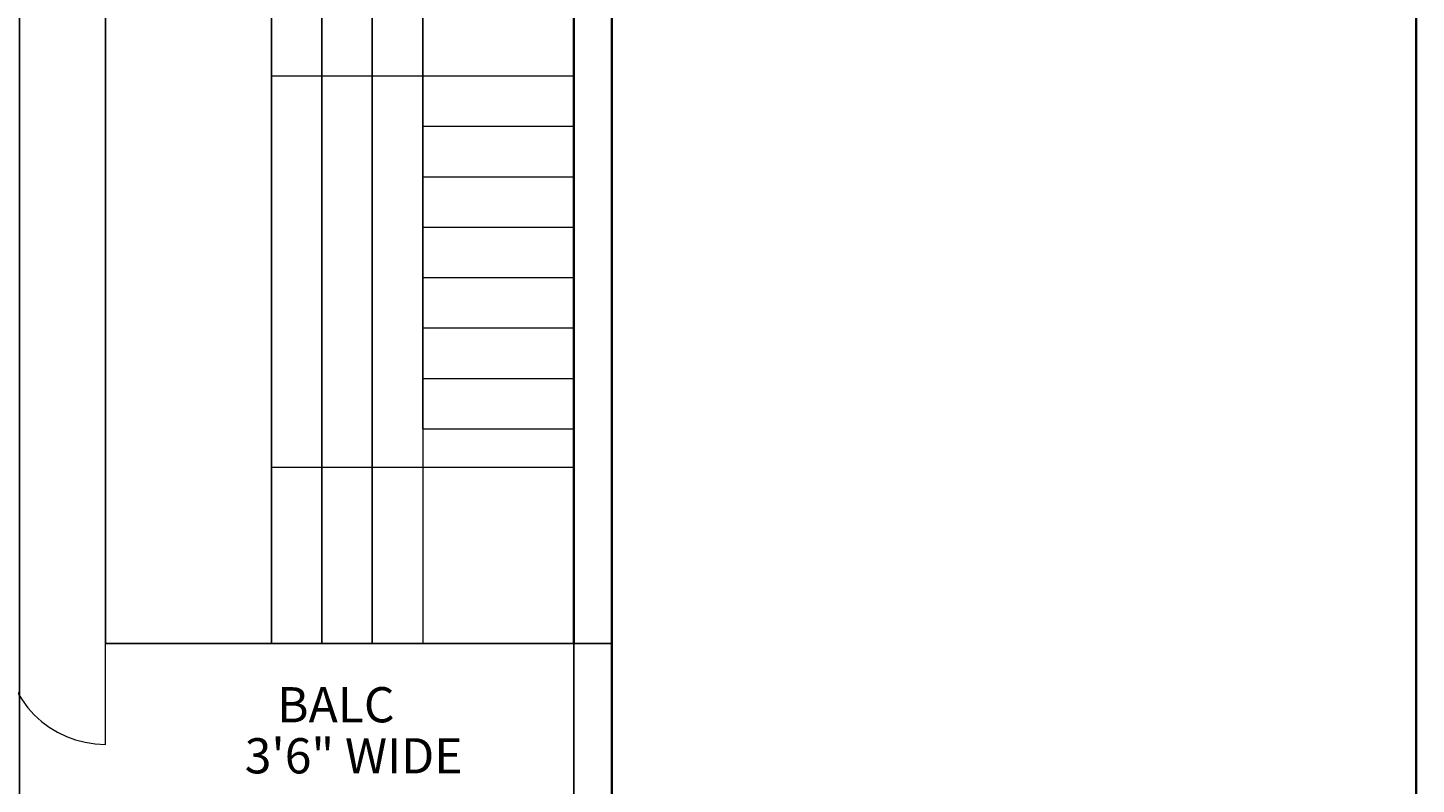
# Model space of a CAD drawing. Units: feet. Extents: x 1654 to 2985, y 1348 to 2230.
# Tile 43 of 53: x 2655 to 2985, y 1532 to 1712. Entities that reach past the tile are written whole.
import ezdxf

# ---------------------------------------------------------------- set-up
doc = ezdxf.new("R2010")
doc.units = ezdxf.units.FT
for name, color, linetype, lineweight in [('A-ANNO-DIMS', 2, 'Continuous', 18), ('A-ANNO-TTLB', 7, 'Continuous', 35), ('A-AREA-IDEN', 7, 'Continuous', 18), ('A-DOOR', 3, 'Continuous', 18), ('A-FLOR', 7, 'Continuous', 25), ('A-FLOR-STRS', 7, 'Continuous', 18), ('A-WALL', 7, 'Continuous', 35)]:
    doc.layers.add(name, color=color, linetype=linetype, lineweight=lineweight)
doc.styles.get("Standard").update_dxf_attribs({"font": 'arial.ttf'})
doc.dimstyles.get("Standard").update_dxf_attribs({"dimtxt": 0.18, "dimasz": 0.18, "dimexe": 0.18, "dimexo": 0.0625, "dimgap": 0.09, "dimtad": 0, "dimtih": 1, "dimtoh": 1, "dimdec": 4, "dimzin": 0, "dimdsep": 46, "dimtxsty": 'Standard', "dimcen": 0.09, "dimadec": 0, "dimazin": 0, "dimtfac": 1, "dimtdec": 4, "dimtofl": 0, "dimtmove": 0, "dimatfit": 3, "dimfxl": 1, "dimtolj": 1, "dimtzin": 0, "dimarcsym": 0})

# ---------------------------------------------------------------- blocks, each defined once
blk = doc.blocks.new('STAIR-RETURN')
for p, q in [((0, 186), (0, 135)), ((36, 186), (36, 0)), ((0, 177), (0, 135)), ((12, 177), (12, 135)), ((12, 177), (12, 135)), ((24, 177), (24, 135)), ((24, 177), (24, 135)), ((72, 135), (0, 135)), ((72, 123), (36, 123)), ((72, 111), (36, 111)), ((72, 99), (36, 99)), ((72, 87), (36, 87)), ((72, 75), (36, 75)), ((72, 63), (36, 63)), ((72, 51), (36, 51)), ((0, 42), (72, 42)), ((0, 42), (0, 0)), ((12, 42), (12, 0)), ((24, 42), (24, 0))]:
    blk.add_line(p, q)
blk = doc.blocks.new('*D82')
at = {"layer": 'A-ANNO-DIMS', "color": 0, "lineweight": -2, "transparency": 16777216}
for p, q in [((2652.71, 2039.19), (2652.71, 1490.62)), ((2784.71, 2039.19), (2784.71, 1490.62)), ((2652.89, 1490.8), (2718.43, 1490.8)), ((2784.53, 1490.8), (2718.99, 1490.8))]:
    blk.add_line(p, q, dxfattribs=at)
at = {"layer": 'A-ANNO-DIMS', "color": 0, "transparency": 16777216}
for points in [[(2652.89, 1490.83), (2652.89, 1490.77), (2652.71, 1490.8)], [(2784.53, 1490.83), (2784.53, 1490.77), (2784.71, 1490.8)]]:
    blk.add_solid(points, dxfattribs=at)
at = {"layer": 'Defpoints', "color": 0, "transparency": 16777216}
for p in [(2652.71, 2039.25), (2784.71, 2039.25), (2784.71, 1490.8)]:
    blk.add_point(p, dxfattribs=at)
at = {"layer": 'A-ANNO-DIMS', "color": 0, "transparency": 16777216, "insert": (2718.71, 1490.8), "char_height": 0.18, "attachment_point": 5}
blk.add_mtext('\\A1;132', dxfattribs=at)
blk = doc.blocks.new('*D84')
at = {"layer": 'A-ANNO-DIMS', "color": 0, "lineweight": -2, "transparency": 16777216}
for p, q in [((2625.24, 1565.32), (2625.24, 2149.88)), ((2625.42, 2149.7), (2649.01, 2149.7)), ((2673.06, 2149.7), (2649.46, 2149.7)), ((2673.24, 1565.32), (2673.24, 2149.88))]:
    blk.add_line(p, q, dxfattribs=at)
at = {"layer": 'A-ANNO-DIMS', "color": 0, "transparency": 16777216}
for points in [[(2625.42, 2149.73), (2625.42, 2149.67), (2625.24, 2149.7)], [(2673.06, 2149.73), (2673.06, 2149.67), (2673.24, 2149.7)]]:
    blk.add_solid(points, dxfattribs=at)
at = {"layer": 'Defpoints', "color": 0, "transparency": 16777216}
for p in [(2673.24, 2149.7), (2625.24, 1565.25), (2673.24, 1565.25)]:
    blk.add_point(p, dxfattribs=at)
at = {"layer": 'A-ANNO-DIMS', "color": 0, "transparency": 16777216, "insert": (2649.24, 2149.7), "char_height": 0.18, "attachment_point": 5}
blk.add_mtext('\\A1;48', dxfattribs=at)
blk = doc.blocks.new('*D85')
at = {"layer": 'A-ANNO-DIMS', "color": 0, "lineweight": -2, "transparency": 16777216}
for p, q in [((2673.24, 1565.32), (2673.24, 2149.88)), ((2673.42, 2149.7), (2692.58, 2149.7)), ((2712.53, 2149.7), (2693.36, 2149.7)), ((2712.71, 1565.32), (2712.71, 2149.88))]:
    blk.add_line(p, q, dxfattribs=at)
at = {"layer": 'A-ANNO-DIMS', "color": 0, "transparency": 16777216}
for points in [[(2673.42, 2149.73), (2673.42, 2149.67), (2673.24, 2149.7)], [(2712.53, 2149.73), (2712.53, 2149.67), (2712.71, 2149.7)]]:
    blk.add_solid(points, dxfattribs=at)
at = {"layer": 'Defpoints', "color": 0, "transparency": 16777216}
for p in [(2712.71, 2149.7), (2673.24, 1565.25), (2712.71, 1565.25)]:
    blk.add_point(p, dxfattribs=at)
at = {"layer": 'A-ANNO-DIMS', "color": 0, "transparency": 16777216, "insert": (2692.97, 2149.7), "char_height": 0.18, "attachment_point": 5}
blk.add_mtext('\\A1;39.47', dxfattribs=at)
blk = doc.blocks.new('*D86')
at = {"layer": 'A-ANNO-DIMS', "color": 0, "lineweight": -2, "transparency": 16777216}
for p, q in [((2748.71, 1616.32), (2748.71, 2149.88)), ((2748.89, 2149.7), (2766.49, 2149.7)), ((2784.53, 2149.7), (2766.92, 2149.7)), ((2784.71, 1607.32), (2784.71, 2149.88))]:
    blk.add_line(p, q, dxfattribs=at)
at = {"layer": 'A-ANNO-DIMS', "color": 0, "transparency": 16777216}
for points in [[(2748.89, 2149.73), (2748.89, 2149.67), (2748.71, 2149.7)], [(2784.53, 2149.73), (2784.53, 2149.67), (2784.71, 2149.7)]]:
    blk.add_solid(points, dxfattribs=at)
at = {"layer": 'Defpoints', "color": 0, "transparency": 16777216}
for p in [(2784.71, 2149.7), (2748.71, 1616.25), (2784.71, 1607.25)]:
    blk.add_point(p, dxfattribs=at)
at = {"layer": 'A-ANNO-DIMS', "color": 0, "transparency": 16777216, "insert": (2766.71, 2149.7), "char_height": 0.18, "attachment_point": 5}
blk.add_mtext('\\A1;36', dxfattribs=at)
blk = doc.blocks.new('*D87')
at = {"layer": 'A-ANNO-DIMS', "color": 0, "lineweight": -2, "transparency": 16777216}
for p, q in [((2724.71, 1565.32), (2724.71, 2149.88)), ((2724.89, 2149.7), (2730.5, 2149.7)), ((2736.53, 2149.7), (2730.92, 2149.7)), ((2736.71, 1565.32), (2736.71, 2149.88))]:
    blk.add_line(p, q, dxfattribs=at)
at = {"layer": 'A-ANNO-DIMS', "color": 0, "transparency": 16777216}
for points in [[(2724.89, 2149.73), (2724.89, 2149.67), (2724.71, 2149.7)], [(2736.53, 2149.73), (2736.53, 2149.67), (2736.71, 2149.7)]]:
    blk.add_solid(points, dxfattribs=at)
at = {"layer": 'Defpoints', "color": 0, "transparency": 16777216}
for p in [(2736.71, 2149.7), (2724.71, 1565.25), (2736.71, 1565.25)]:
    blk.add_point(p, dxfattribs=at)
at = {"layer": 'A-ANNO-DIMS', "color": 0, "transparency": 16777216, "insert": (2730.71, 2149.7), "char_height": 0.18, "attachment_point": 5}
blk.add_mtext('\\A1;12', dxfattribs=at)

msp = doc.modelspace()

# ---------------------------------------------------------------- linework, layer by layer
at = {"layer": 'A-ANNO-TTLB'}
msp.add_lwpolyline([(1654.1997, 2230.0267), (2985.175, 2230.0267), (2985.175, 1348.1324), (1654.1997, 1348.1324)], close=True, dxfattribs=at)
at = {"layer": 'A-DOOR'}
msp.add_line((2673.2353, 1541.2549), (2673.2353, 1565.2549), dxfattribs=at)
msp.add_arc((2673.2353, 1565.2549), 24, 180, 270, dxfattribs=at)
at = {"layer": 'A-FLOR'}
msp.add_line((2673.2353, 1565.2549), (2793.7058, 1565.2549), dxfattribs=at)
at = {"layer": 'A-WALL'}
for p, q in [((2793.7058, 1886.2549), (2793.7058, 1523.2549)), ((2784.7058, 1742.2549), (2784.7058, 1565.2549))]:
    msp.add_line(p, q, dxfattribs=at)

# ---------------------------------------------------------------- block references
at = {"layer": 'A-FLOR-STRS'}
msp.add_blockref('STAIR-RETURN', (2712.7054, 1565.255), dxfattribs=at)

# ---------------------------------------------------------------- texts
at = {"layer": 'A-AREA-IDEN'}
for s, p in [('BALC', (2714.0307, 1546.4962)), ('3\'6" WIDE', (2706.3476, 1534.3486))]:
    msp.add_text(s, height=8.38114, dxfattribs=at).set_placement(p)

# ---------------------------------------------------------------- dimensions: what is measured, and where the dimension line sits
at = {"layer": 'A-ANNO-DIMS'}
for base, p1, p2, override, picture, middle in [((2673.2353, 2149.7049), (2625.2353, 1565.2549), (2673.2353, 1565.2549), {"dimdec": 0, "dimlfac": 1, "dimrnd": 0, "dimzin": 0, "dimdsep": 46, "dimlunit": 2}, '*D84', (2649.2353, 2149.7049)), ((2712.7058, 2149.7049), (2673.2353, 1565.2549), (2712.7058, 1565.2549), {"dimdec": 2, "dimlfac": 1, "dimrnd": 0, "dimzin": 0, "dimdsep": 46, "dimlunit": 2}, '*D85', (2692.9706, 2149.7049)), ((2736.7058, 2149.7049), (2724.7058, 1565.2549), (2736.7058, 1565.2549), {"dimdec": 0, "dimlfac": 1, "dimrnd": 0, "dimzin": 0, "dimdsep": 46, "dimlunit": 2}, '*D87', (2730.7058, 2149.7049)), ((2784.7058, 2149.7049), (2748.7058, 1616.2549), (2784.7058, 1607.2549), {"dimdec": 0, "dimlfac": 1, "dimrnd": 0, "dimzin": 0, "dimdsep": 46, "dimlunit": 2}, '*D86', (2766.7058, 2149.7049)), ((2784.7058, 1490.8049), (2652.7058, 2039.2549), (2784.7058, 2039.2549), {"dimdec": 0, "dimlfac": 1, "dimrnd": 0, "dimzin": 0, "dimdsep": 46, "dimlunit": 2}, '*D82', (2718.7058, 1490.8049))]:
    dim = msp.add_linear_dim(base=base, p1=p1, p2=p2, dimstyle='Standard', override=override, dxfattribs=at)
    dim.commit()
    dim.dimension.update_dxf_attribs({"geometry": picture, "text_midpoint": middle})

doc.saveas('drawing.dxf')
